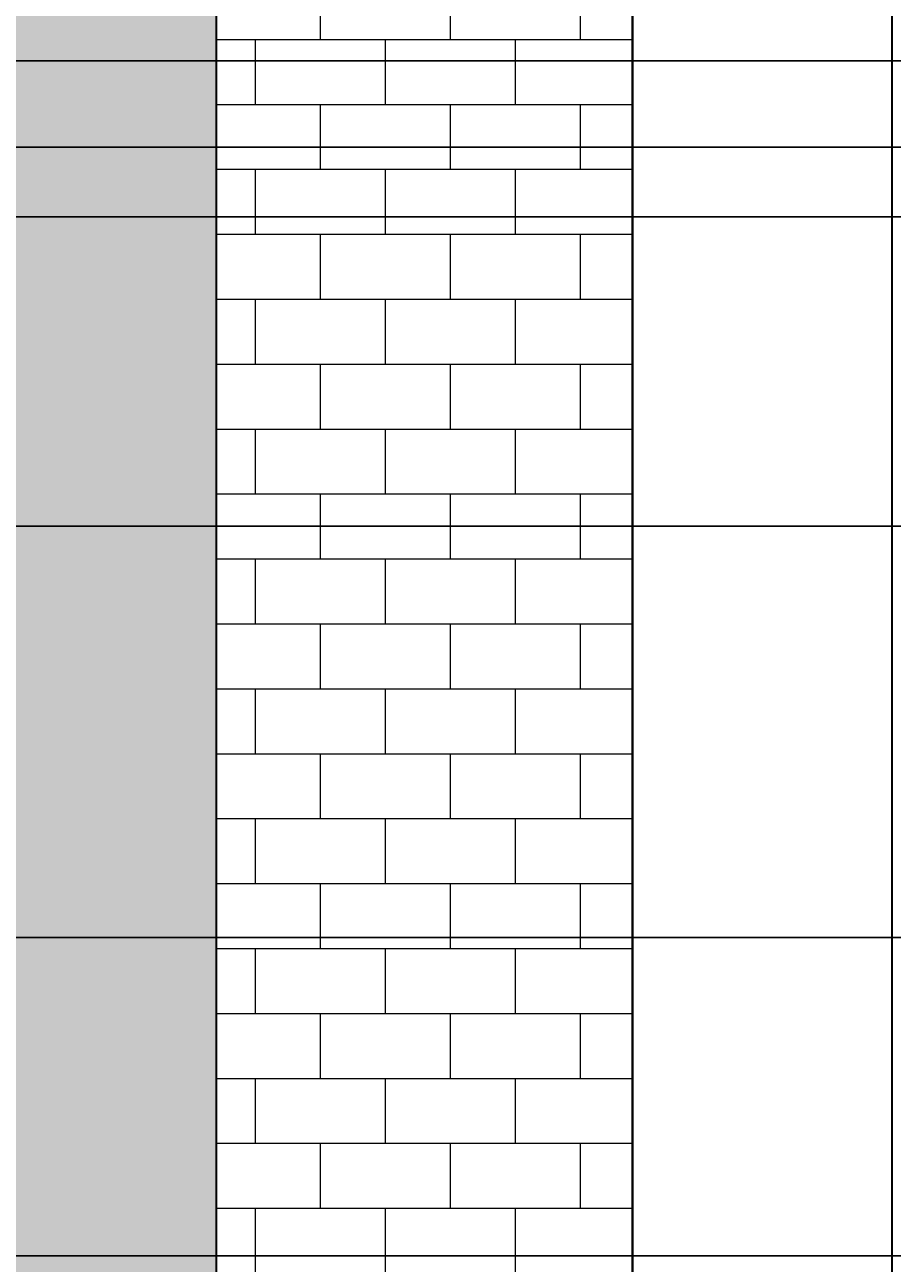
# Model space of a CAD drawing. Units: inches. Extents: x -13 to 809, y 112 to 656.
# Tile 47 of 55: x 521 to 621, y 324 to 467. Entities that reach past the tile are written whole.
import ezdxf

# ---------------------------------------------------------------- set-up
doc = ezdxf.new("R2010")
doc.units = ezdxf.units.IN
doc.header["$MEASUREMENT"] = 0
for name, color, linetype, lineweight in [('A-ANNO-DIMS', 2, 'Continuous', 18), ('A-ELEV', 7, 'Continuous', 35), ('A-ELEV-PATT', 8, 'Continuous', 13)]:
    doc.layers.add(name, color=color, linetype=linetype, lineweight=lineweight)
doc.styles.get("Standard").update_dxf_attribs({"font": 'arial.ttf'})
doc.dimstyles.get("Standard").update_dxf_attribs({"dimtxt": 0.625, "dimasz": 0.18, "dimexe": 0.18, "dimexo": 0.0625, "dimgap": 0.09, "dimtad": 0, "dimtih": 1, "dimtoh": 1, "dimdec": 4, "dimzin": 0, "dimdsep": 46, "dimlunit": 4, "dimtxsty": 'Standard', "dimcen": 0.09, "dimadec": 0, "dimazin": 0, "dimtfac": 1, "dimtdec": 4, "dimtofl": 0, "dimtmove": 0, "dimatfit": 3, "dimfxl": 1, "dimtolj": 1, "dimtzin": 0, "dimarcsym": 0})

# ---------------------------------------------------------------- blocks, each defined once
blk = doc.blocks.new('*D46')
at = {"layer": 'A-ANNO-DIMS', "color": 0, "lineweight": -2, "transparency": 16777216}
for p, q in [((160.98, 408.79), (807.77, 408.79)), ((807.59, 408.61), (807.59, 367.07)), ((807.59, 324.7), (807.59, 366.25)), ((160.98, 324.52), (807.77, 324.52))]:
    blk.add_line(p, q, dxfattribs=at)
at = {"layer": 'A-ANNO-DIMS', "color": 0, "transparency": 16777216}
for points in [[(807.56, 408.61), (807.62, 408.61), (807.59, 408.79)], [(807.56, 324.7), (807.62, 324.7), (807.59, 324.52)]]:
    blk.add_solid(points, dxfattribs=at)
at = {"layer": 'Defpoints', "color": 0, "transparency": 16777216}
for p in [(160.92, 408.79), (807.59, 408.79), (160.92, 324.52)]:
    blk.add_point(p, dxfattribs=at)
at = {"layer": 'A-ANNO-DIMS', "color": 0, "transparency": 16777216, "insert": (807.59, 366.66), "char_height": 0.625, "attachment_point": 5}
blk.add_mtext('\\A1;84.27', dxfattribs=at)
blk = doc.blocks.new('*D47')
at = {"layer": 'A-ANNO-DIMS', "color": 0, "lineweight": -2, "transparency": 16777216}
for p, q in [((275.78, 408.79), (807.77, 408.79)), ((807.59, 408.61), (807.59, 385.45)), ((807.59, 361.47), (807.59, 384.63)), ((275.78, 361.29), (807.77, 361.29))]:
    blk.add_line(p, q, dxfattribs=at)
at = {"layer": 'A-ANNO-DIMS', "color": 0, "transparency": 16777216}
for points in [[(807.56, 408.61), (807.62, 408.61), (807.59, 408.79)], [(807.56, 361.47), (807.62, 361.47), (807.59, 361.29)]]:
    blk.add_solid(points, dxfattribs=at)
at = {"layer": 'Defpoints', "color": 0, "transparency": 16777216}
for p in [(275.71, 408.79), (807.59, 408.79), (275.71, 361.29)]:
    blk.add_point(p, dxfattribs=at)
at = {"layer": 'A-ANNO-DIMS', "color": 0, "transparency": 16777216, "insert": (807.59, 385.04), "char_height": 0.625, "attachment_point": 5}
blk.add_mtext('\\A1;47.5', dxfattribs=at)
blk = doc.blocks.new('*D48')
at = {"layer": 'A-ANNO-DIMS', "color": 0, "lineweight": -2, "transparency": 16777216}
for p, q in [((319.57, 444.52), (807.77, 444.52)), ((807.59, 444.34), (807.59, 384.93)), ((807.59, 324.7), (807.59, 384.11)), ((319.57, 324.52), (807.77, 324.52))]:
    blk.add_line(p, q, dxfattribs=at)
at = {"layer": 'A-ANNO-DIMS', "color": 0, "transparency": 16777216}
for points in [[(807.56, 444.34), (807.62, 444.34), (807.59, 444.52)], [(807.56, 324.7), (807.62, 324.7), (807.59, 324.52)]]:
    blk.add_solid(points, dxfattribs=at)
at = {"layer": 'Defpoints', "color": 0, "transparency": 16777216}
for p in [(319.51, 444.52), (807.59, 444.52), (319.51, 324.52)]:
    blk.add_point(p, dxfattribs=at)
at = {"layer": 'A-ANNO-DIMS', "color": 0, "transparency": 16777216, "insert": (807.59, 384.52), "char_height": 0.625, "attachment_point": 5}
blk.add_mtext('\\A1;120', dxfattribs=at)
blk = doc.blocks.new('*D104')
at = {"layer": 'A-ANNO-DIMS', "color": 0, "lineweight": -2, "transparency": 16777216}
for p, q in [((337.57, 462.52), (807.77, 462.52)), ((807.59, 462.34), (807.59, 457.95)), ((807.59, 452.74), (807.59, 457.13)), ((319.76, 452.56), (807.77, 452.56))]:
    blk.add_line(p, q, dxfattribs=at)
at = {"layer": 'A-ANNO-DIMS', "color": 0, "transparency": 16777216}
for points in [[(807.56, 462.34), (807.62, 462.34), (807.59, 462.52)], [(807.56, 452.74), (807.62, 452.74), (807.59, 452.56)]]:
    blk.add_solid(points, dxfattribs=at)
at = {"layer": 'Defpoints', "color": 0, "transparency": 16777216}
for p in [(337.51, 462.52), (319.7, 452.56), (807.59, 452.56)]:
    blk.add_point(p, dxfattribs=at)
at = {"layer": 'A-ANNO-DIMS', "color": 0, "transparency": 16777216, "insert": (807.59, 457.54), "char_height": 0.625, "attachment_point": 5}
blk.add_mtext('\\A1;9.957', dxfattribs=at)
blk = doc.blocks.new('*D105')
at = {"layer": 'A-ANNO-DIMS', "color": 0, "lineweight": -2, "transparency": 16777216}
for p, q in [((319.76, 452.56), (807.77, 452.56)), ((807.59, 452.38), (807.59, 448.95)), ((807.59, 444.7), (807.59, 448.13)), ((319.57, 444.52), (807.77, 444.52))]:
    blk.add_line(p, q, dxfattribs=at)
at = {"layer": 'A-ANNO-DIMS', "color": 0, "transparency": 16777216}
for points in [[(807.56, 452.38), (807.62, 452.38), (807.59, 452.56)], [(807.56, 444.7), (807.62, 444.7), (807.59, 444.52)]]:
    blk.add_solid(points, dxfattribs=at)
at = {"layer": 'Defpoints', "color": 0, "transparency": 16777216}
for p in [(319.7, 452.56), (319.51, 444.52), (807.59, 444.52)]:
    blk.add_point(p, dxfattribs=at)
at = {"layer": 'A-ANNO-DIMS', "color": 0, "transparency": 16777216, "insert": (807.59, 448.54), "char_height": 0.625, "attachment_point": 5}
blk.add_mtext('\\A1;8.043', dxfattribs=at)

msp = doc.modelspace()

# ---------------------------------------------------------------- hatches: boundary and pattern name
at = {"layer": 'A-ELEV-PATT'}
h = msp.add_hatch(dxfattribs=at)
h.set_pattern_fill('BRICK', color=256, scale=30)
h.paths.add_polyline_path([(591.008, 558.5199), (341.4072, 558.5199), (341.4072, 524.281), (542.9617, 524.281), (542.9617, 288.4508), (341.4072, 288.4508), (341.4072, 250.8429), (591.008, 250.8429)])
h = msp.add_hatch(dxfattribs=at)
h.set_pattern_fill('CROSS', color=256, scale=9.7)
h.paths.add_polyline_path([(542.9617, 524.281), (442.1845, 524.281), (442.1845, 288.4508), (542.9617, 288.4508)])
h.paths.add_polyline_path([(471.0998, 470.8765), (471.0998, 498.1452), (510.462, 498.1452), (510.462, 470.8765)], flags=16)
h.paths.add_polyline_path([(473.0998, 472.8765), (473.0998, 496.1452), (508.462, 496.1452), (508.462, 472.8765)], flags=0)
h.paths.add_polyline_path([(471.0998, 442.128), (510.462, 442.128), (510.462, 414.8594), (471.0998, 414.8594)], flags=16)
h.paths.add_polyline_path([(473.0998, 440.128), (508.462, 440.128), (508.462, 416.8594), (473.0998, 416.8594)], flags=0)
h.paths.add_polyline_path([(471.0998, 385.2491), (510.462, 385.2491), (510.462, 357.9804), (471.0998, 357.9804)], flags=16)
h.paths.add_polyline_path([(473.0998, 383.2491), (508.462, 383.2491), (508.462, 359.9804), (473.0998, 359.9804)], flags=0)
h.paths.add_polyline_path([(471.0998, 340.4353), (510.462, 340.4353), (510.462, 313.1667), (471.0998, 313.1667)], flags=16)
h.paths.add_polyline_path([(473.0998, 338.4353), (508.462, 338.4353), (508.462, 315.1667), (473.0998, 315.1667)], flags=0)

# ---------------------------------------------------------------- linework, layer by layer
at = {"layer": 'A-ELEV'}
for p, q in [((591.008, 209.8635), (591.008, 558.5199)), ((621.008, 209.8635), (621.008, 558.5199))]:
    msp.add_line(p, q, dxfattribs=at)
for points in [[(341.4072, 558.5199), (591.008, 558.5199), (591.008, 250.8429), (341.4072, 250.8429)], [(341.4072, 524.281), (542.9617, 524.281), (542.9617, 288.4508), (341.4072, 288.4508)]]:
    msp.add_lwpolyline(points, close=True, dxfattribs=at)

# ---------------------------------------------------------------- dimensions: what is measured, and where the dimension line sits
at = {"layer": 'A-ANNO-DIMS'}
for base, p1, p2, override, picture, middle in [((807.5888, 452.5629), (337.5074, 462.5199), (319.7004, 452.5629), {"dimdec": 3, "dimlfac": 1, "dimrnd": 0, "dimzin": 0, "dimdsep": 46, "dimlunit": 2}, '*D104', (807.5888, 457.5414)), ((807.5888, 444.5199), (319.7004, 452.5629), (319.5074, 444.5199), {"dimdec": 3, "dimlfac": 1, "dimrnd": 0, "dimzin": 0, "dimdsep": 46, "dimlunit": 2}, '*D105', (807.5888, 448.5414)), ((807.5888, 444.5199), (319.5074, 324.5199), (319.5074, 444.5199), {"dimdec": 0, "dimlfac": 1, "dimrnd": 0, "dimzin": 0, "dimdsep": 46, "dimlunit": 2}, '*D48', (807.5888, 384.5199)), ((807.5888, 408.7939), (160.9184, 324.5199), (160.9184, 408.7939), {"dimdec": 2, "dimlfac": 1, "dimrnd": 0, "dimzin": 0, "dimdsep": 46, "dimlunit": 2}, '*D46', (807.5888, 366.6569)), ((807.5888, 408.7939), (275.7145, 361.2915), (275.7145, 408.7939), {"dimdec": 1, "dimlfac": 1, "dimrnd": 0, "dimzin": 0, "dimdsep": 46, "dimlunit": 2}, '*D47', (807.5888, 385.0427))]:
    dim = msp.add_linear_dim(base=base, p1=p1, p2=p2, angle=90, dimstyle='Standard', override=override, dxfattribs=at)
    dim.commit()
    dim.dimension.update_dxf_attribs({"geometry": picture, "text_midpoint": middle})

doc.saveas('drawing.dxf')
